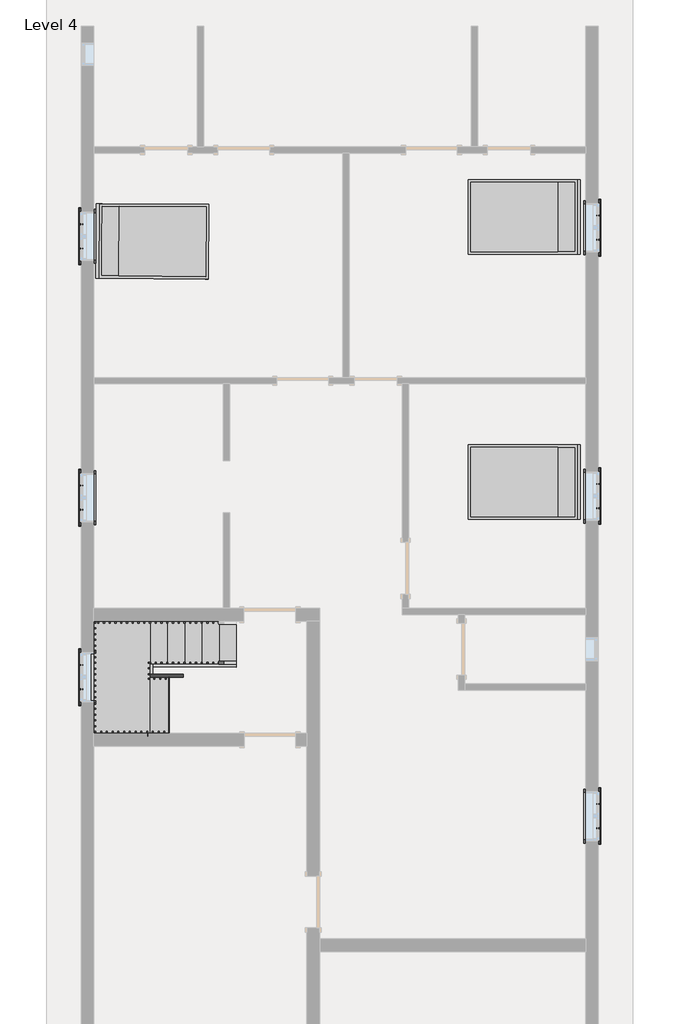
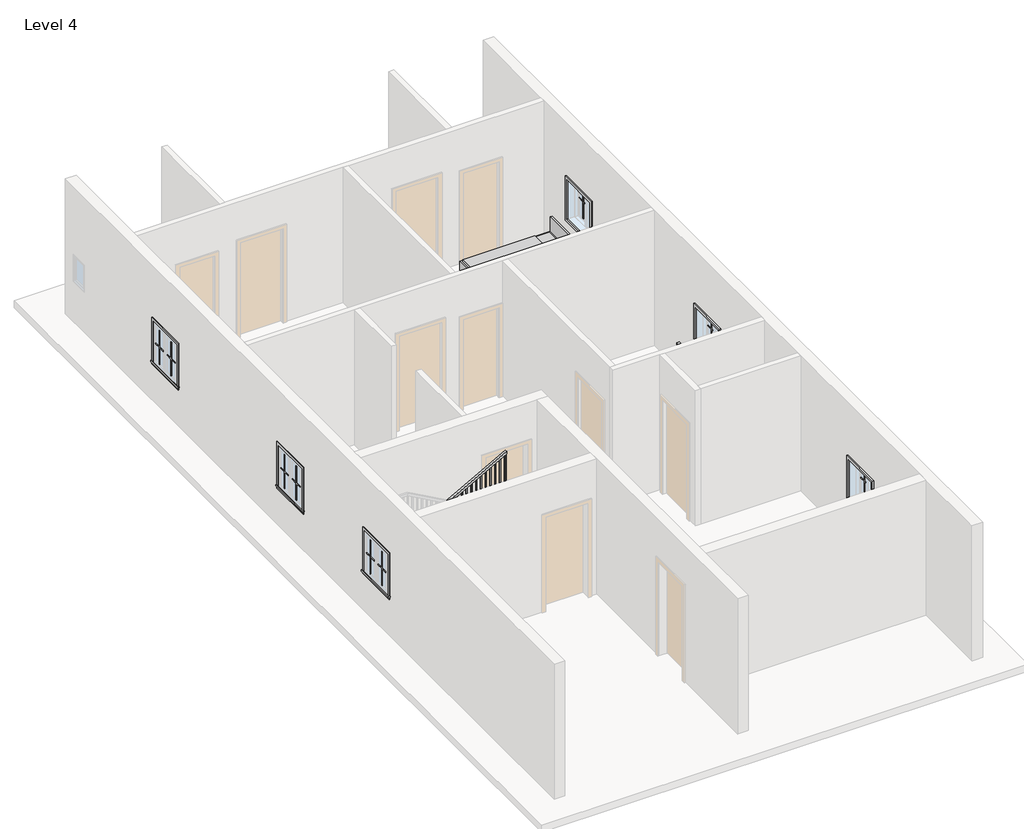
# One storey, part 3 of 3: 24 proxies, 6 members, 3 furniture elements, 1 railing, 1 stair flight.
"""IFC4 building model written with IfcOpenShell, lengths in millimetres."""

from ifc_helpers import new_model, si_unit, frame, origin, place, context, project, spatial, polyline, outline, extrude, faceted_brep, transform, mapped, element, save
from components import muntin_pattern_2x2_muntin_pattern_2x2_b3fe6957, muntin_pattern_2x2_muntin_pattern_2x2_3e0ecaf2, trim_window_exterior_flat_with_sill_41619996, trim_window_interior_flat_picture_frame_51c85655, bed_17739_bed_17739_15c61121, stair_flight_58fc4bcf

model = new_model("IFC4")

# Units and contexts
model_context = context("Model", 3, world=origin())
ifc_project = project(units=[si_unit("LENGTHUNIT", "METRE", prefix="MILLI")], contexts=[model_context])

# Site, building, storey
site = spatial("IfcSite", under=ifc_project)
building = spatial("IfcBuilding", under=site)
storey = spatial("IfcBuildingStorey", under=building, Name="Level 4", Elevation=6400.8)

# Proxies
placement = place(None, origin())
muntin_pattern_2x2_muntin_pattern_2x2_shape = muntin_pattern_2x2_muntin_pattern_2x2_b3fe6957(model_context)
element("IfcBuildingElementProxy", 1, Name="Muntin Pattern_2x2 : Muntin Pattern_2x2", ObjectType="Muntin Pattern_2x2 : Muntin Pattern_2x2", at=placement, inside=storey, context=model_context, shape_type="MappedRepresentation", body=[
    mapped(muntin_pattern_2x2_muntin_pattern_2x2_shape, transform((3307.2334916, 6850.4197267, 7385.05), x_axis=(0.0, -1.0, 0.0), y_axis=(1.0, 0.0, 0.0), z_axis=(0.0, 0.0, 1.0))),
])
element("IfcBuildingElementProxy", 2, Name="Muntin Pattern_2x2 : Muntin Pattern_2x2", ObjectType="Muntin Pattern_2x2 : Muntin Pattern_2x2", at=placement, inside=storey, context=model_context, shape_type="MappedRepresentation", body=[
    mapped(muntin_pattern_2x2_muntin_pattern_2x2_shape, transform((3307.2334916, 2106.9697267, 7385.05), x_axis=(0.0, -1.0, 0.0), y_axis=(1.0, 0.0, 0.0), z_axis=(0.0, 0.0, 1.0))),
])
element("IfcBuildingElementProxy", 3, Name="Muntin Pattern_2x2 : Muntin Pattern_2x2", ObjectType="Muntin Pattern_2x2 : Muntin Pattern_2x2", at=placement, inside=storey, context=model_context, shape_type="MappedRepresentation", body=[
    mapped(muntin_pattern_2x2_muntin_pattern_2x2_shape, transform((-5817.7165084, 6269.3947267, 7385.05), x_axis=(0.0, 1.0, 0.0), y_axis=(-1.0, 0.0, 0.0), z_axis=(0.0, 0.0, 1.0))),
])
element("IfcBuildingElementProxy", 4, Name="Muntin Pattern_2x2 : Muntin Pattern_2x2", ObjectType="Muntin Pattern_2x2 : Muntin Pattern_2x2", at=placement, inside=storey, context=model_context, shape_type="MappedRepresentation", body=[
    mapped(muntin_pattern_2x2_muntin_pattern_2x2_shape, transform((-5817.7165084, 1649.7697267, 7385.05), x_axis=(0.0, 1.0, 0.0), y_axis=(-1.0, 0.0, 0.0), z_axis=(0.0, 0.0, 1.0))),
])
element("IfcBuildingElementProxy", 5, Name="Muntin Pattern_2x2 : Muntin Pattern_2x2", ObjectType="Muntin Pattern_2x2 : Muntin Pattern_2x2", at=placement, inside=storey, context=model_context, shape_type="MappedRepresentation", body=[
    mapped(muntin_pattern_2x2_muntin_pattern_2x2_shape, transform((3307.2334916, -3547.7052733, 7385.05), x_axis=(0.0, -1.0, 0.0), y_axis=(1.0, 0.0, 0.0), z_axis=(0.0, 0.0, 1.0))),
])
element("IfcBuildingElementProxy", 6, Name="Muntin Pattern_2x2 : Muntin Pattern_2x2", ObjectType="Muntin Pattern_2x2 : Muntin Pattern_2x2", at=placement, inside=storey, context=model_context, shape_type="MappedRepresentation", body=[
    mapped(muntin_pattern_2x2_muntin_pattern_2x2_shape, transform((-5817.7165084, -1522.0552733, 7385.05), x_axis=(0.0, 1.0, 0.0), y_axis=(-1.0, 0.0, 0.0), z_axis=(0.0, 0.0, 1.0))),
])
muntin_pattern_2x2_muntin_pattern_2x2_2_shape = muntin_pattern_2x2_muntin_pattern_2x2_3e0ecaf2(model_context)
element("IfcBuildingElementProxy", 7, Name="Muntin Pattern_2x2 : Muntin Pattern_2x2", ObjectType="Muntin Pattern_2x2 : Muntin Pattern_2x2", at=placement, inside=storey, context=model_context, shape_type="MappedRepresentation", body=[
    mapped(muntin_pattern_2x2_muntin_pattern_2x2_2_shape, transform((3307.2334916, 6421.7947267, 7385.05), x_axis=(0.0, 1.0, 0.0), y_axis=(-1.0, 0.0, 0.0), z_axis=(0.0, 0.0, 1.0))),
])
element("IfcBuildingElementProxy", 8, Name="Muntin Pattern_2x2 : Muntin Pattern_2x2", ObjectType="Muntin Pattern_2x2 : Muntin Pattern_2x2", at=placement, inside=storey, context=model_context, shape_type="MappedRepresentation", body=[
    mapped(muntin_pattern_2x2_muntin_pattern_2x2_2_shape, transform((3307.2334916, 1678.3447267, 7385.05), x_axis=(0.0, 1.0, 0.0), y_axis=(-1.0, 0.0, 0.0), z_axis=(0.0, 0.0, 1.0))),
])
element("IfcBuildingElementProxy", 9, Name="Muntin Pattern_2x2 : Muntin Pattern_2x2", ObjectType="Muntin Pattern_2x2 : Muntin Pattern_2x2", at=placement, inside=storey, context=model_context, shape_type="MappedRepresentation", body=[
    mapped(muntin_pattern_2x2_muntin_pattern_2x2_2_shape, transform((-5817.7165084, 6698.0197267, 7385.05), x_axis=(0.0, -1.0, 0.0), y_axis=(1.0, 0.0, 0.0), z_axis=(0.0, 0.0, 1.0))),
])
element("IfcBuildingElementProxy", 10, Name="Muntin Pattern_2x2 : Muntin Pattern_2x2", ObjectType="Muntin Pattern_2x2 : Muntin Pattern_2x2", at=placement, inside=storey, context=model_context, shape_type="MappedRepresentation", body=[
    mapped(muntin_pattern_2x2_muntin_pattern_2x2_2_shape, transform((-5817.7165084, 2078.3947267, 7385.05), x_axis=(0.0, -1.0, 0.0), y_axis=(1.0, 0.0, 0.0), z_axis=(0.0, 0.0, 1.0))),
])
element("IfcBuildingElementProxy", 11, Name="Muntin Pattern_2x2 : Muntin Pattern_2x2", ObjectType="Muntin Pattern_2x2 : Muntin Pattern_2x2", at=placement, inside=storey, context=model_context, shape_type="MappedRepresentation", body=[
    mapped(muntin_pattern_2x2_muntin_pattern_2x2_2_shape, transform((3307.2334916, -3976.3302733, 7385.05), x_axis=(0.0, 1.0, 0.0), y_axis=(-1.0, 0.0, 0.0), z_axis=(0.0, 0.0, 1.0))),
])
element("IfcBuildingElementProxy", 12, Name="Muntin Pattern_2x2 : Muntin Pattern_2x2", ObjectType="Muntin Pattern_2x2 : Muntin Pattern_2x2", at=placement, inside=storey, context=model_context, shape_type="MappedRepresentation", body=[
    mapped(muntin_pattern_2x2_muntin_pattern_2x2_2_shape, transform((-5817.7165084, -1093.4302733, 7385.05), x_axis=(0.0, -1.0, 0.0), y_axis=(1.0, 0.0, 0.0), z_axis=(0.0, 0.0, 1.0))),
])
trim_window_exterior_flat_with_sill_shape = trim_window_exterior_flat_with_sill_41619996(model_context)
element("IfcBuildingElementProxy", 13, Name="Trim-Window-Exterior-Flat : with Sill", ObjectType="Trim-Window-Exterior-Flat : with Sill", at=placement, inside=storey, context=model_context, shape_type="MappedRepresentation", body=[
    mapped(trim_window_exterior_flat_with_sill_shape, transform((3316.7584916, 6636.1072267, 8229.6), x_axis=(0.0, 1.0, 0.0), y_axis=(0.0, 0.0, 1.0), z_axis=(1.0, 0.0, 0.0))),
])
element("IfcBuildingElementProxy", 14, Name="Trim-Window-Exterior-Flat : with Sill", ObjectType="Trim-Window-Exterior-Flat : with Sill", at=placement, inside=storey, context=model_context, shape_type="MappedRepresentation", body=[
    mapped(trim_window_exterior_flat_with_sill_shape, transform((3316.7584916, 1892.6572267, 8229.6), x_axis=(0.0, 1.0, 0.0), y_axis=(0.0, 0.0, 1.0), z_axis=(1.0, 0.0, 0.0))),
])
element("IfcBuildingElementProxy", 15, Name="Trim-Window-Exterior-Flat : with Sill", ObjectType="Trim-Window-Exterior-Flat : with Sill", at=placement, inside=storey, context=model_context, shape_type="MappedRepresentation", body=[
    mapped(trim_window_exterior_flat_with_sill_shape, transform((-5827.2415084, 6483.7072267, 8229.6), x_axis=(0.0, -1.0, 0.0), y_axis=(0.0, 0.0, 1.0), z_axis=(-1.0, 0.0, 0.0))),
])
element("IfcBuildingElementProxy", 16, Name="Trim-Window-Exterior-Flat : with Sill", ObjectType="Trim-Window-Exterior-Flat : with Sill", at=placement, inside=storey, context=model_context, shape_type="MappedRepresentation", body=[
    mapped(trim_window_exterior_flat_with_sill_shape, transform((-5827.2415084, 1864.0822267, 8229.6), x_axis=(0.0, -1.0, 0.0), y_axis=(0.0, 0.0, 1.0), z_axis=(-1.0, 0.0, 0.0))),
])
element("IfcBuildingElementProxy", 17, Name="Trim-Window-Exterior-Flat : with Sill", ObjectType="Trim-Window-Exterior-Flat : with Sill", at=placement, inside=storey, context=model_context, shape_type="MappedRepresentation", body=[
    mapped(trim_window_exterior_flat_with_sill_shape, transform((3316.7584916, -3762.0177733, 8229.6), x_axis=(0.0, 1.0, 0.0), y_axis=(0.0, 0.0, 1.0), z_axis=(1.0, 0.0, 0.0))),
])
element("IfcBuildingElementProxy", 18, Name="Trim-Window-Exterior-Flat : with Sill", ObjectType="Trim-Window-Exterior-Flat : with Sill", at=placement, inside=storey, context=model_context, shape_type="MappedRepresentation", body=[
    mapped(trim_window_exterior_flat_with_sill_shape, transform((-5827.2415084, -1307.7427733, 8229.6), x_axis=(0.0, -1.0, 0.0), y_axis=(0.0, 0.0, 1.0), z_axis=(-1.0, 0.0, 0.0))),
])
trim_window_interior_flat_picture_frame_shape = trim_window_interior_flat_picture_frame_51c85655(model_context)
element("IfcBuildingElementProxy", 19, Name="Trim-Window-Interior-Flat : Picture Frame", ObjectType="Trim-Window-Interior-Flat : Picture Frame", at=placement, inside=storey, context=model_context, shape_type="MappedRepresentation", body=[
    mapped(trim_window_interior_flat_picture_frame_shape, transform((3088.1584916, 6636.1072267, 8229.6), x_axis=(0.0, -1.0, 0.0), y_axis=(0.0, 0.0, 1.0), z_axis=(-1.0, 0.0, 0.0))),
])
element("IfcBuildingElementProxy", 20, Name="Trim-Window-Interior-Flat : Picture Frame", ObjectType="Trim-Window-Interior-Flat : Picture Frame", at=placement, inside=storey, context=model_context, shape_type="MappedRepresentation", body=[
    mapped(trim_window_interior_flat_picture_frame_shape, transform((3088.1584916, 1892.6572267, 8229.6), x_axis=(0.0, -1.0, 0.0), y_axis=(0.0, 0.0, 1.0), z_axis=(-1.0, 0.0, 0.0))),
])
element("IfcBuildingElementProxy", 21, Name="Trim-Window-Interior-Flat : Picture Frame", ObjectType="Trim-Window-Interior-Flat : Picture Frame", at=placement, inside=storey, context=model_context, shape_type="MappedRepresentation", body=[
    mapped(trim_window_interior_flat_picture_frame_shape, transform((-5598.6415084, 6483.7072267, 8229.6), x_axis=(0.0, 1.0, 0.0), y_axis=(0.0, 0.0, 1.0), z_axis=(1.0, 0.0, 0.0))),
])
element("IfcBuildingElementProxy", 22, Name="Trim-Window-Interior-Flat : Picture Frame", ObjectType="Trim-Window-Interior-Flat : Picture Frame", at=placement, inside=storey, context=model_context, shape_type="MappedRepresentation", body=[
    mapped(trim_window_interior_flat_picture_frame_shape, transform((-5598.6415084, 1864.0822267, 8229.6), x_axis=(0.0, 1.0, 0.0), y_axis=(0.0, 0.0, 1.0), z_axis=(1.0, 0.0, 0.0))),
])
element("IfcBuildingElementProxy", 23, Name="Trim-Window-Interior-Flat : Picture Frame", ObjectType="Trim-Window-Interior-Flat : Picture Frame", at=placement, inside=storey, context=model_context, shape_type="MappedRepresentation", body=[
    mapped(trim_window_interior_flat_picture_frame_shape, transform((3088.1584916, -3762.0177733, 8229.6), x_axis=(0.0, -1.0, 0.0), y_axis=(0.0, 0.0, 1.0), z_axis=(-1.0, 0.0, 0.0))),
])
element("IfcBuildingElementProxy", 24, Name="Trim-Window-Interior-Flat : Picture Frame", ObjectType="Trim-Window-Interior-Flat : Picture Frame", at=placement, inside=storey, context=model_context, shape_type="MappedRepresentation", body=[
    mapped(trim_window_interior_flat_picture_frame_shape, transform((-5598.6415084, -1307.7427733, 8229.6), x_axis=(0.0, 1.0, 0.0), y_axis=(0.0, 0.0, 1.0), z_axis=(1.0, 0.0, 0.0))),
])

# Furniture
bed_17739_bed_17739_shape = bed_17739_bed_17739_15c61121(model_context)
element("IfcFurniture", 25, ObjectType="Bed_17739 : Bed_17739", at=placement, inside=storey, context=model_context, shape_type="MappedRepresentation", body=[
    mapped(bed_17739_bed_17739_shape, transform((-4543.6279345, 6394.2844586, 6400.8), x_axis=(0.007593038844487308, 0.9999711724650396, 0.0), y_axis=(-0.9999711724650396, 0.007593038844487308, 0.0), z_axis=(0.0, 0.0, 1.0))),
])
element("IfcFurniture", 26, ObjectType="Bed_17739 : Bed_17739", at=placement, inside=storey, context=model_context, shape_type="MappedRepresentation", body=[
    mapped(bed_17739_bed_17739_shape, transform((1983.2584916, 6826.6072267, 6400.8), x_axis=(0.0, -1.0, 0.0), y_axis=(1.0, 0.0, 0.0), z_axis=(0.0, 0.0, 1.0))),
])
element("IfcFurniture", 27, ObjectType="Bed_17739 : Bed_17739", at=placement, inside=storey, context=model_context, shape_type="MappedRepresentation", body=[
    mapped(bed_17739_bed_17739_shape, transform((1983.2584916, 2140.3072267, 6400.8), x_axis=(0.0, -1.0, 0.0), y_axis=(1.0, 0.0, 0.0), z_axis=(0.0, 0.0, 1.0))),
])

# Members
element("IfcMember", 28, ObjectType="Stringer - 2\" Width", at=placement, inside=storey, context=model_context, shape_type="SweptSolid", body=[
    extrude(outline(polyline([(6400.8, -3084.0415084), (6608.3983948, -3084.0415084), (7426.8428392, -4557.2415084), (7078.1641651, -4557.2415084), (6400.8, -3337.9860112), (6400.8, -3084.0415084)])), frame((0.0, -1127.4758739, 0.0), z_axis=(0.0, 1.0, 0.0), x_axis=(0.0, 0.0, 1.0)), (0.0, 0.0, 1.0), 50.8),
])
element("IfcMember", 29, ObjectType="Stringer - 2\" Width", at=placement, inside=storey, context=model_context, shape_type="SweptSolid", body=[
    extrude(outline(polyline([(-4608.0415084, -1076.6758739), (-4557.2415084, -1076.6758739), (-4557.2415084, -1256.9427733), (-4608.0415084, -1256.9427733), (-4608.0415084, -1076.6758739)])), frame((0.0, 0.0, 7188.2), z_axis=(0.0, 0.0, 1.0), x_axis=(1.0, 0.0, 0.0)), (0.0, 0.0, 1.0), 304.8),
])
element("IfcMember", 30, ObjectType="Stringer - 2\" Width", at=placement, inside=storey, context=model_context, shape_type="SweptSolid", body=[
    extrude(outline(polyline([(7624.3983948, -4608.0415084), (7275.7197207, -4608.0415084), (8122.3863873, -3084.0415084), (8471.0650614, -3084.0415084), (7624.3983948, -4608.0415084)])), frame((0.0, -1307.7427733, 0.0), z_axis=(0.0, 1.0, 0.0), x_axis=(0.0, 0.0, 1.0)), (0.0, 0.0, 1.0), 50.8),
])
element("IfcMember", 31, ObjectType="Stringer - 2\" Width", at=placement, inside=storey, context=model_context, shape_type="SweptSolid", body=[
    extrude(outline(polyline([(6400.8, -3084.0415084), (6608.3983948, -3084.0415084), (7493.0, -4676.3243978), (7493.0, -5303.9460112), (6400.8, -3337.9860112), (6400.8, -3084.0415084)])), frame((0.0, -317.1427733, 0.0), z_axis=(0.0, 1.0, 0.0), x_axis=(0.0, 0.0, 1.0)), (0.0, 0.0, 1.0), 50.8),
])
element("IfcMember", 32, ObjectType="Stringer - 2\" Width", at=placement, inside=storey, context=model_context, shape_type="SweptSolid", body=[
    extrude(outline(polyline([(-5649.4415084, -266.3427733), (-5598.6415084, -266.3427733), (-5598.6415084, -2298.3427733), (-5649.4415084, -2298.3427733), (-5649.4415084, -266.3427733)])), frame((0.0, 0.0, 7188.2), z_axis=(0.0, 0.0, 1.0), x_axis=(1.0, 0.0, 0.0)), (0.0, 0.0, 1.0), 304.8),
])
element("IfcMember", 33, ObjectType="Stringer - 2\" Width", at=placement, inside=storey, context=model_context, shape_type="SweptSolid", body=[
    extrude(outline(polyline([(7188.2, -4765.5770056), (8122.3863873, -3084.0415084), (8471.0650614, -3084.0415084), (7188.2, -5393.198619), (7188.2, -4765.5770056)])), frame((0.0, -2349.1427733, 0.0), z_axis=(0.0, 1.0, 0.0), x_axis=(0.0, 0.0, 1.0)), (0.0, 0.0, 1.0), 50.8),
])

# Railing
element("IfcRailing", 34, ObjectType="Handrail - Rectangular", at=placement, inside=storey, context=model_context, shape_type="SolidModel", body=[
    faceted_brep([(-3084.0415084, -1076.6758739, 7484.5333333), (-3084.0415084, -1076.6758739, 7426.420221), (-3084.0415084, -1025.8758739, 7426.420221), (-3084.0415084, -1025.8758739, 7484.5333333), (-4531.8415084, -1076.6758739, 8288.8666667), (-4582.6415084, -1076.6758739, 8258.9757765), (-4582.6415084, -1025.8758739, 8258.9757765), (-4531.8415084, -1025.8758739, 8288.8666667), (-4531.8415084, -1076.6758739, 8331.2), (-4582.6415084, -1076.6758739, 8280.4), (-4582.6415084, -1025.8758739, 8280.4), (-4531.8415084, -1025.8758739, 8331.2), (-4608.0415084, -1076.6758739, 8331.2), (-4608.0415084, -1076.6758739, 8280.4), (-4658.8415084, -1025.8758739, 8280.4), (-4658.8415084, -1025.8758739, 8331.2), (-4608.0415084, -1152.8758739, 8331.2), (-4608.0415084, -1152.8758739, 8280.4), (-4658.8415084, -1152.8758739, 8280.4), (-4658.8415084, -1152.8758739, 8331.2), (-4608.0415084, -1231.5427733, 8331.2), (-4608.0415084, -1282.3427733, 8280.4), (-4658.8415084, -1282.3427733, 8280.4), (-4658.8415084, -1231.5427733, 8331.2), (-4608.0415084, -1231.5427733, 8542.8666667), (-4608.0415084, -1282.3427733, 8492.0666667), (-4658.8415084, -1282.3427733, 8492.0666667), (-4658.8415084, -1231.5427733, 8542.8666667), (-4608.0415084, -1307.7427733, 8542.8666667), (-4608.0415084, -1307.7427733, 8492.0666667), (-4658.8415084, -1358.5427733, 8492.0666667), (-4658.8415084, -1358.5427733, 8542.8666667), (-4531.8415084, -1307.7427733, 8542.8666667), (-4518.6779062, -1307.7427733, 8492.0666667), (-4518.6779062, -1358.5427733, 8492.0666667), (-4531.8415084, -1358.5427733, 8542.8666667), (-3084.0415084, -1307.7427733, 9347.2), (-3084.0415084, -1358.5427733, 9347.2), (-3084.0415084, -1358.5427733, 9289.0868876), (-3084.0415084, -1307.7427733, 9289.0868876)], [[[0, 1, 2, 3]], [[1, 0, 4, 5]], [[2, 1, 5, 6]], [[3, 2, 6, 7]], [[0, 3, 7, 4]], [[5, 4, 8, 9]], [[6, 5, 9, 10]], [[7, 6, 10, 11]], [[4, 7, 11, 8]], [[9, 8, 12, 13]], [[10, 9, 13, 14]], [[11, 10, 14, 15]], [[8, 11, 15, 12]], [[13, 12, 16, 17]], [[14, 13, 17, 18]], [[15, 14, 18, 19]], [[12, 15, 19, 16]], [[17, 16, 20, 21]], [[18, 17, 21, 22]], [[19, 18, 22, 23]], [[16, 19, 23, 20]], [[21, 20, 24, 25]], [[22, 21, 25, 26]], [[23, 22, 26, 27]], [[20, 23, 27, 24]], [[25, 24, 28, 29]], [[26, 25, 29, 30]], [[27, 26, 30, 31]], [[24, 27, 31, 28]], [[29, 28, 32, 33]], [[30, 29, 33, 34]], [[31, 30, 34, 35]], [[28, 31, 35, 32]], [[36, 37, 38, 39]], [[33, 32, 36, 39]], [[34, 33, 39, 38]], [[35, 34, 38, 37]], [[32, 35, 37, 36]]]),
    extrude(outline(polyline([(9269.6841099, -3118.9665084), (8263.4666667, -3118.9665084), (8263.4666667, -3099.9165084), (9280.2674432, -3099.9165084), (9269.6841099, -3118.9665084)])), frame((0.0, -1342.6677733, 0.0), z_axis=(0.0, 1.0, 0.0), x_axis=(0.0, 0.0, 1.0)), (0.0, 0.0, 1.0), 19.05),
    extrude(outline(polyline([(9213.2396654, -3220.5665084), (8263.4666667, -3220.5665084), (8263.4666667, -3201.5165084), (9223.8229988, -3201.5165084), (9213.2396654, -3220.5665084)])), frame((0.0, -1342.6677733, 0.0), z_axis=(0.0, 1.0, 0.0), x_axis=(0.0, 0.0, 1.0)), (0.0, 0.0, 1.0), 19.05),
    extrude(outline(polyline([(9156.795221, -3322.1665084), (8263.4666667, -3322.1665084), (8263.4666667, -3303.1165084), (9167.3785543, -3303.1165084), (9156.795221, -3322.1665084)])), frame((0.0, -1342.6677733, 0.0), z_axis=(0.0, 1.0, 0.0), x_axis=(0.0, 0.0, 1.0)), (0.0, 0.0, 1.0), 19.05),
    extrude(outline(polyline([(9100.3507765, -3423.7665084), (8094.1333333, -3423.7665084), (8094.1333333, -3404.7165084), (9110.9341099, -3404.7165084), (9100.3507765, -3423.7665084)])), frame((0.0, -1342.6677733, 0.0), z_axis=(0.0, 1.0, 0.0), x_axis=(0.0, 0.0, 1.0)), (0.0, 0.0, 1.0), 19.05),
    extrude(outline(polyline([(9043.9063321, -3525.3665084), (8094.1333333, -3525.3665084), (8094.1333333, -3506.3165084), (9054.4896654, -3506.3165084), (9043.9063321, -3525.3665084)])), frame((0.0, -1342.6677733, 0.0), z_axis=(0.0, 1.0, 0.0), x_axis=(0.0, 0.0, 1.0)), (0.0, 0.0, 1.0), 19.05),
    extrude(outline(polyline([(8987.4618876, -3626.9665084), (8094.1333333, -3626.9665084), (8094.1333333, -3607.9165084), (8998.045221, -3607.9165084), (8987.4618876, -3626.9665084)])), frame((0.0, -1342.6677733, 0.0), z_axis=(0.0, 1.0, 0.0), x_axis=(0.0, 0.0, 1.0)), (0.0, 0.0, 1.0), 19.05),
    extrude(outline(polyline([(8931.0174432, -3728.5665084), (7924.8, -3728.5665084), (7924.8, -3709.5165084), (8941.6007765, -3709.5165084), (8931.0174432, -3728.5665084)])), frame((0.0, -1342.6677733, 0.0), z_axis=(0.0, 1.0, 0.0), x_axis=(0.0, 0.0, 1.0)), (0.0, 0.0, 1.0), 19.05),
    extrude(outline(polyline([(8874.5729988, -3830.1665084), (7924.8, -3830.1665084), (7924.8, -3811.1165084), (8885.1563321, -3811.1165084), (8874.5729988, -3830.1665084)])), frame((0.0, -1342.6677733, 0.0), z_axis=(0.0, 1.0, 0.0), x_axis=(0.0, 0.0, 1.0)), (0.0, 0.0, 1.0), 19.05),
    extrude(outline(polyline([(8818.1285543, -3931.7665084), (7924.8, -3931.7665084), (7924.8, -3912.7165084), (8828.7118876, -3912.7165084), (8818.1285543, -3931.7665084)])), frame((0.0, -1342.6677733, 0.0), z_axis=(0.0, 1.0, 0.0), x_axis=(0.0, 0.0, 1.0)), (0.0, 0.0, 1.0), 19.05),
    extrude(outline(polyline([(8761.6841099, -4033.3665084), (7755.4666667, -4033.3665084), (7755.4666667, -4014.3165084), (8772.2674432, -4014.3165084), (8761.6841099, -4033.3665084)])), frame((0.0, -1342.6677733, 0.0), z_axis=(0.0, 1.0, 0.0), x_axis=(0.0, 0.0, 1.0)), (0.0, 0.0, 1.0), 19.05),
    extrude(outline(polyline([(8705.2396654, -4134.9665084), (7755.4666667, -4134.9665084), (7755.4666667, -4115.9165084), (8715.8229988, -4115.9165084), (8705.2396654, -4134.9665084)])), frame((0.0, -1342.6677733, 0.0), z_axis=(0.0, 1.0, 0.0), x_axis=(0.0, 0.0, 1.0)), (0.0, 0.0, 1.0), 19.05),
    extrude(outline(polyline([(8648.795221, -4236.5665084), (7755.4666667, -4236.5665084), (7755.4666667, -4217.5165084), (8659.3785543, -4217.5165084), (8648.795221, -4236.5665084)])), frame((0.0, -1342.6677733, 0.0), z_axis=(0.0, 1.0, 0.0), x_axis=(0.0, 0.0, 1.0)), (0.0, 0.0, 1.0), 19.05),
    extrude(outline(polyline([(8592.3507765, -4338.1665084), (7586.1333333, -4338.1665084), (7586.1333333, -4319.1165084), (8602.9341099, -4319.1165084), (8592.3507765, -4338.1665084)])), frame((0.0, -1342.6677733, 0.0), z_axis=(0.0, 1.0, 0.0), x_axis=(0.0, 0.0, 1.0)), (0.0, 0.0, 1.0), 19.05),
    extrude(outline(polyline([(8535.9063321, -4439.7665084), (7586.1333333, -4439.7665084), (7586.1333333, -4420.7165084), (8546.4896654, -4420.7165084), (8535.9063321, -4439.7665084)])), frame((0.0, -1342.6677733, 0.0), z_axis=(0.0, 1.0, 0.0), x_axis=(0.0, 0.0, 1.0)), (0.0, 0.0, 1.0), 19.05),
    extrude(outline(polyline([(8479.4618876, -4541.3665084), (7586.1333333, -4541.3665084), (7586.1333333, -4522.3165084), (8490.045221, -4522.3165084), (8479.4618876, -4541.3665084)])), frame((0.0, -1342.6677733, 0.0), z_axis=(0.0, 1.0, 0.0), x_axis=(0.0, 0.0, 1.0)), (0.0, 0.0, 1.0), 19.05),
    extrude(outline(polyline([(-4623.9165084, -1244.9508739), (-4623.9165084, -1264.0008739), (-4642.9665084, -1264.0008739), (-4642.9665084, -1244.9508739), (-4623.9165084, -1244.9508739)])), frame((0.0, 0.0, 7416.8), z_axis=(0.0, 0.0, 1.0), x_axis=(1.0, 0.0, 0.0)), (0.0, 0.0, 1.0), 1075.2666667),
    extrude(outline(polyline([(-4623.9165084, -1143.3508739), (-4623.9165084, -1162.4008739), (-4642.9665084, -1162.4008739), (-4642.9665084, -1143.3508739), (-4623.9165084, -1143.3508739)])), frame((0.0, 0.0, 7416.8), z_axis=(0.0, 0.0, 1.0), x_axis=(1.0, 0.0, 0.0)), (0.0, 0.0, 1.0), 863.6),
    extrude(outline(polyline([(-4598.5165084, -1060.8008739), (-4617.5665084, -1060.8008739), (-4617.5665084, -1041.7508739), (-4598.5165084, -1041.7508739), (-4598.5165084, -1060.8008739)])), frame((0.0, 0.0, 7416.8), z_axis=(0.0, 0.0, 1.0), x_axis=(1.0, 0.0, 0.0)), (0.0, 0.0, 1.0), 863.6),
    extrude(outline(polyline([(8221.9341099, -4515.9665084), (7247.4666667, -4515.9665084), (7247.4666667, -4496.9165084), (8211.3507765, -4496.9165084), (8221.9341099, -4515.9665084)])), frame((0.0, -1060.8008739, 0.0), z_axis=(0.0, 1.0, 0.0), x_axis=(0.0, 0.0, 1.0)), (0.0, 0.0, 1.0), 19.05),
    extrude(outline(polyline([(8165.4896654, -4414.3665084), (7247.4666667, -4414.3665084), (7247.4666667, -4395.3165084), (8154.9063321, -4395.3165084), (8165.4896654, -4414.3665084)])), frame((0.0, -1060.8008739, 0.0), z_axis=(0.0, 1.0, 0.0), x_axis=(0.0, 0.0, 1.0)), (0.0, 0.0, 1.0), 19.05),
    extrude(outline(polyline([(8109.045221, -4312.7665084), (7247.4666667, -4312.7665084), (7247.4666667, -4293.7165084), (8098.4618876, -4293.7165084), (8109.045221, -4312.7665084)])), frame((0.0, -1060.8008739, 0.0), z_axis=(0.0, 1.0, 0.0), x_axis=(0.0, 0.0, 1.0)), (0.0, 0.0, 1.0), 19.05),
    extrude(outline(polyline([(8052.6007765, -4211.1665084), (7078.1333333, -4211.1665084), (7078.1333333, -4192.1165084), (8042.0174432, -4192.1165084), (8052.6007765, -4211.1665084)])), frame((0.0, -1060.8008739, 0.0), z_axis=(0.0, 1.0, 0.0), x_axis=(0.0, 0.0, 1.0)), (0.0, 0.0, 1.0), 19.05),
    extrude(outline(polyline([(7996.1563321, -4109.5665084), (7078.1333333, -4109.5665084), (7078.1333333, -4090.5165084), (7985.5729988, -4090.5165084), (7996.1563321, -4109.5665084)])), frame((0.0, -1060.8008739, 0.0), z_axis=(0.0, 1.0, 0.0), x_axis=(0.0, 0.0, 1.0)), (0.0, 0.0, 1.0), 19.05),
    extrude(outline(polyline([(7939.7118876, -4007.9665084), (7078.1333333, -4007.9665084), (7078.1333333, -3988.9165084), (7929.1285543, -3988.9165084), (7939.7118876, -4007.9665084)])), frame((0.0, -1060.8008739, 0.0), z_axis=(0.0, 1.0, 0.0), x_axis=(0.0, 0.0, 1.0)), (0.0, 0.0, 1.0), 19.05),
    extrude(outline(polyline([(7883.2674432, -3906.3665084), (6908.8, -3906.3665084), (6908.8, -3887.3165084), (7872.6841099, -3887.3165084), (7883.2674432, -3906.3665084)])), frame((0.0, -1060.8008739, 0.0), z_axis=(0.0, 1.0, 0.0), x_axis=(0.0, 0.0, 1.0)), (0.0, 0.0, 1.0), 19.05),
    extrude(outline(polyline([(7826.8229988, -3804.7665084), (6908.8, -3804.7665084), (6908.8, -3785.7165084), (7816.2396654, -3785.7165084), (7826.8229988, -3804.7665084)])), frame((0.0, -1060.8008739, 0.0), z_axis=(0.0, 1.0, 0.0), x_axis=(0.0, 0.0, 1.0)), (0.0, 0.0, 1.0), 19.05),
    extrude(outline(polyline([(7770.3785543, -3703.1665084), (6908.8, -3703.1665084), (6908.8, -3684.1165084), (7759.795221, -3684.1165084), (7770.3785543, -3703.1665084)])), frame((0.0, -1060.8008739, 0.0), z_axis=(0.0, 1.0, 0.0), x_axis=(0.0, 0.0, 1.0)), (0.0, 0.0, 1.0), 19.05),
    extrude(outline(polyline([(7713.9341099, -3601.5665084), (6739.4666667, -3601.5665084), (6739.4666667, -3582.5165084), (7703.3507765, -3582.5165084), (7713.9341099, -3601.5665084)])), frame((0.0, -1060.8008739, 0.0), z_axis=(0.0, 1.0, 0.0), x_axis=(0.0, 0.0, 1.0)), (0.0, 0.0, 1.0), 19.05),
    extrude(outline(polyline([(7657.4896654, -3499.9665084), (6739.4666667, -3499.9665084), (6739.4666667, -3480.9165084), (7646.9063321, -3480.9165084), (7657.4896654, -3499.9665084)])), frame((0.0, -1060.8008739, 0.0), z_axis=(0.0, 1.0, 0.0), x_axis=(0.0, 0.0, 1.0)), (0.0, 0.0, 1.0), 19.05),
    extrude(outline(polyline([(7601.045221, -3398.3665084), (6739.4666667, -3398.3665084), (6739.4666667, -3379.3165084), (7590.4618876, -3379.3165084), (7601.045221, -3398.3665084)])), frame((0.0, -1060.8008739, 0.0), z_axis=(0.0, 1.0, 0.0), x_axis=(0.0, 0.0, 1.0)), (0.0, 0.0, 1.0), 19.05),
    extrude(outline(polyline([(7544.6007765, -3296.7665084), (6570.1333333, -3296.7665084), (6570.1333333, -3277.7165084), (7534.0174432, -3277.7165084), (7544.6007765, -3296.7665084)])), frame((0.0, -1060.8008739, 0.0), z_axis=(0.0, 1.0, 0.0), x_axis=(0.0, 0.0, 1.0)), (0.0, 0.0, 1.0), 19.05),
    extrude(outline(polyline([(7488.1563321, -3195.1665084), (6570.1333333, -3195.1665084), (6570.1333333, -3176.1165084), (7477.5729988, -3176.1165084), (7488.1563321, -3195.1665084)])), frame((0.0, -1060.8008739, 0.0), z_axis=(0.0, 1.0, 0.0), x_axis=(0.0, 0.0, 1.0)), (0.0, 0.0, 1.0), 19.05),
    extrude(outline(polyline([(-4623.9165084, -1323.6177733), (-4623.9165084, -1342.6677733), (-4642.9665084, -1342.6677733), (-4642.9665084, -1323.6177733), (-4623.9165084, -1323.6177733)])), frame((0.0, 0.0, 7416.8), z_axis=(0.0, 0.0, 1.0), x_axis=(1.0, 0.0, 0.0)), (0.0, 0.0, 1.0), 1075.2666667),
    extrude(outline(polyline([(-4623.9165084, -1060.8008739), (-4642.9665084, -1060.8008739), (-4642.9665084, -1041.7508739), (-4623.9165084, -1041.7508739), (-4623.9165084, -1060.8008739)])), frame((0.0, 0.0, 7416.8), z_axis=(0.0, 0.0, 1.0), x_axis=(1.0, 0.0, 0.0)), (0.0, 0.0, 1.0), 863.6),
    extrude(outline(polyline([(9278.5035543, -3103.0915084), (8263.4666667, -3103.0915084), (8263.4666667, -3084.0415084), (9289.0868876, -3084.0415084), (9278.5035543, -3103.0915084)])), frame((0.0, -1342.6677733, 0.0), z_axis=(0.0, 1.0, 0.0), x_axis=(0.0, 0.0, 1.0)), (0.0, 0.0, 1.0), 19.05),
    extrude(outline(polyline([(7437.0035543, -3103.0915084), (6570.1333333, -3103.0915084), (6570.1333333, -3084.0415084), (7426.420221, -3084.0415084), (7437.0035543, -3103.0915084)])), frame((0.0, -1060.8008739, 0.0), z_axis=(0.0, 1.0, 0.0), x_axis=(0.0, 0.0, 1.0)), (0.0, 0.0, 1.0), 19.05),
])

# Stair flight
stair_flight_shape = stair_flight_58fc4bcf(model_context)
element("IfcStairFlight", 35, ObjectType="2\" Tread 1\" Nosing 1/4\" Riser", at=placement, inside=storey, context=model_context, shape_type="MappedRepresentation", body=[
    mapped(stair_flight_shape, transform((0.0, 0.0, 0.0), x_axis=(1.0, 0.0, 0.0), y_axis=(0.0, 1.0, 0.0), z_axis=(0.0, 0.0, 1.0))),
])

save(model, "model.ifc")

# Revit data of these elements
# Type "Muntin Pattern_2x2 : Muntin Pattern_2x2"
#   Width [instance default] = 4' - 0"
#   Thickness = 0' - 0 1/2"
#   Height [instance default] = 4' - 0"
#   Distance = 0' - 0 3/4"
#   Interior Material [instance default] = none
#   Exterior Material [instance default] = none
#   Default Elevation = 0
# Type "Trim-Window-Exterior-Flat : with Sill"
#   Trim Width = 0' - 2 1/4"
#   Trim Thickness_Picture Frame = 0' - 1 1/4"
#   Trim Thickness_with Sill = 0' - 0 3/4"
#   Sill Thickness = 0' - 1 1/4"
#   Opening Width [instance default] = 2' - 0"
#   Opening Height [instance default] = 3' - 0"
#   Default Elevation = 4' - 0"
#   Sill = yes
#   Picture Frame = no
#   Trim Material [instance default] = none
# Type "Trim-Window-Interior-Flat : Picture Frame"
#   Trim Thickness_Picture Frame = 0' - 1 1/4"
#   Trim Width = 0' - 2 1/4"
#   Trim Thickness_with Sill = 0' - 0 3/4"
#   Sill Thickness = 0' - 1 1/4"
#   Opening Width [instance default] = 2' - 0"
#   Opening Height [instance default] = 3' - 0"
#   Default Elevation = 4' - 0"
#   Sill = no
#   Picture Frame = yes
#   Trim Material [instance default] = none
# Type "Bed_17739 : Bed_17739"
#   Default Elevation = 0
# Type "Handrail - Rectangular"
#   Assembly Code = "C2010400"
#   built-in parameter 1008612 = 0.0416667 (stored number, unit not read)
#   built-in parameter 1008611 = 0.0416667 (stored number, unit not read)
#   built-in parameter 1008609 = 0.333333 (stored number, unit not read)
#   built-in parameter 1008604 = 0.166667 (stored number, unit not read)
#   built-in parameter 1008603 = 0.166667 (stored number, unit not read)
#   Railing Height = 3' - 0"
#   built-in parameter 1008630 = 2
#   built-in parameter 1008610 = 2
#   built-in parameter 1008618 = Baluster - Square : 3/4"
# Elements 1, 2, 3, 4, 5, 6, 7, 8, 9, 10, 11, 12 (IfcBuildingElementProxy, "Muntin Pattern_2x2 : Muntin Pattern_2x2")
#   Width = 0' - 11 5/8"
#   Height = 2' - 6 1/2"
#   Interior Material = Wood - Stained
#   Exterior Material = Clad - White
#   Phase Created = New Construction
#   Materials on its faces: "Clad - White", "Wood - Stained"
# Elements 13, 14, 15, 16, 17, 18 (IfcBuildingElementProxy, "Trim-Window-Exterior-Flat : with Sill")
#   Opening Width = 2' - 10"
#   Opening Height = 3' - 0"
#   Trim Material = Clad - White
#   Phase Created = New Construction
#   Materials on its faces: "Clad - White"
# Elements 19, 20, 21, 22, 23, 24 (IfcBuildingElementProxy, "Trim-Window-Interior-Flat : Picture Frame")
#   Opening Width = 2' - 10"
#   Opening Height = 3' - 0"
#   Trim Material = Wood - Stained
#   Phase Created = New Construction
#   Materials on its faces: "Wood - Stained"
# Elements 25, 26, 27 (IfcFurniture, "Bed_17739 : Bed_17739")
#   Phase Created = New Construction
#   Materials on its faces: "legs", "sheets", "bed frame", "Blanket"
# Elements 28, 29, 30, 31, 32, 33 (IfcMember, "Stringer - 2\" Width")
#   Phase Created = New Construction
# Element 34 (IfcRailing, "Handrail - Rectangular")
#   Phase Created = New Construction
# Element 35 (IfcStairFlight, "2\" Tread 1\" Nosing 1/4\" Riser")
#   Phase Created = New Construction
# Materials
#   "Clad - White": class "Wood", colour RGB 242 242 238, transparency 0, Cost = 0
#   "Wood - Stained": class "Wood", colour RGB 224 178 126, transparency 0, Cost = 0
#   "legs": colour RGB 90 73 37, transparency 0, Cost = 0
#   "sheets": colour RGB 200 195 176, transparency 0, Cost = 0
#   "bed frame": colour RGB 90 73 37, transparency 0, Cost = 0
#   "Blanket": class "System", colour RGB 59 0 1, transparency 0, Cost = 0
